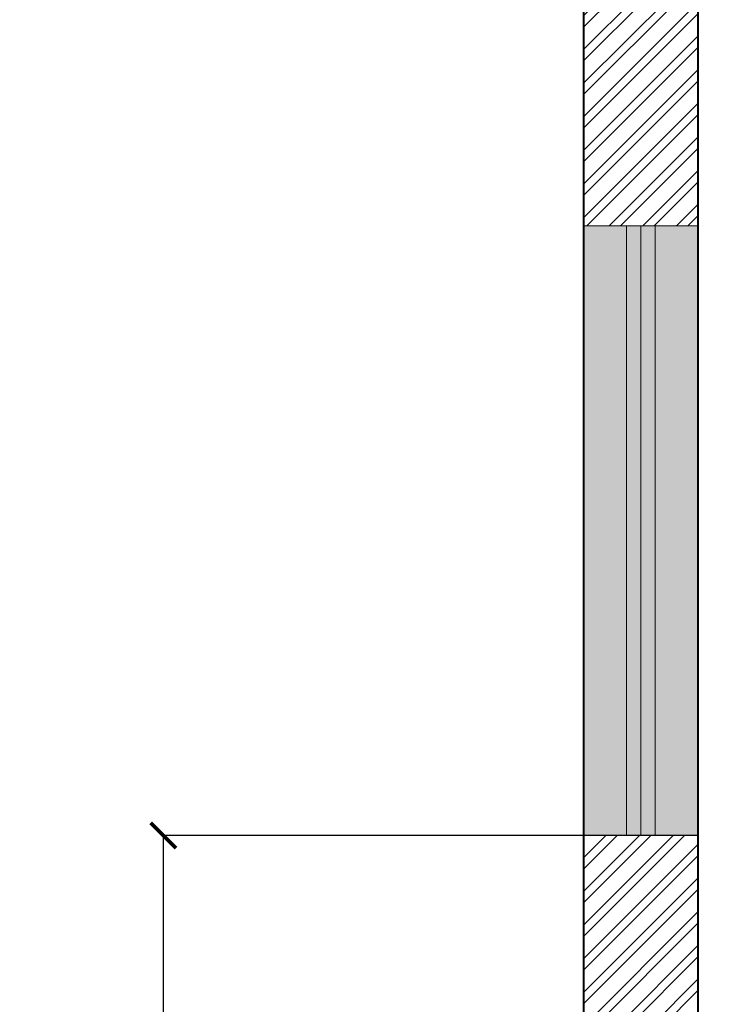
# Model space of a CAD drawing. Units: inches. Extents: x 528 to 2520, y -151 to 1354.
# Tile 17 of 41: x 1079 to 1136, y 1151 to 1228. Entities that reach past the tile are written whole.
import ezdxf

# ---------------------------------------------------------------- set-up
doc = ezdxf.new("R2010")
doc.units = ezdxf.units.IN
doc.header["$MEASUREMENT"] = 0
for name, color, linetype, lineweight in [('A-ANNO-DIMS', 2, 'Continuous', 18), ('A-WALL-PATT', 6, 'Continuous', 13), ('walls', 7, 'Continuous', 40), ('WINDOWS', 2, 'Continuous', 20)]:
    doc.layers.add(name, color=color, linetype=linetype, lineweight=lineweight)
doc.layers.add('A-GLAZ-PATT', color=152, linetype='Continuous', lineweight=13, true_color=0x2776bb)
doc.styles.get("Standard").update_dxf_attribs({"font": 'arial.ttf'})
doc.dimstyles.get("Standard").update_dxf_attribs({"dimtxt": 6, "dimasz": 2, "dimexe": 0.18, "dimexo": 0.0625, "dimgap": 0.09, "dimtad": 0, "dimtih": 1, "dimtoh": 1, "dimdec": 1, "dimzin": 0, "dimdsep": 46, "dimlunit": 3, "dimtxsty": 'Standard', "dimblk": 'ARCHTICK', "dimcen": 0.09, "dimadec": 0, "dimazin": 0, "dimtfac": 1, "dimtdec": 1, "dimtofl": 0, "dimtmove": 0, "dimatfit": 3, "dimfxl": 1, "dimtolj": 1, "dimtzin": 0, "dimarcsym": 0})

# ---------------------------------------------------------------- blocks, each defined once
blk = doc.blocks.new('WINDOW-48x9-PLAN')
for p, q in [((0, 5.632), (48, 5.632)), ((0, 4.5), (48, 4.5)), ((0, 3.368), (48, 3.368))]:
    blk.add_line(p, q)
blk.add_lwpolyline([(0, 9), (48, 9), (48, 0), (0, 0)], close=True)
blk = doc.blocks.new('_ArchTick')
at = {"color": 0, "linetype": 'ByBlock', "const_width": 0.15}
blk.add_lwpolyline([(-0.5, -0.5), (0.5, 0.5)], dxfattribs=at)
blk = doc.blocks.new('*D99')
at = {"layer": 'A-ANNO-DIMS', "color": 0, "lineweight": -2, "transparency": 16777216}
for p, q in [((1132.821, 1163.855), (1090.603, 1163.855)), ((1090.783, 1163.855), (1090.783, 1126.132)), ((1090.783, 1082.103), (1090.783, 1119.826)), ((1132.821, 1082.103), (1090.603, 1082.103))]:
    blk.add_line(p, q, dxfattribs=at)
at = {"layer": 'Defpoints', "color": 0, "transparency": 16777216}
for p in [(1132.883, 1163.855), (1090.783, 1082.103), (1132.883, 1082.103)]:
    blk.add_point(p, dxfattribs=at)
at = {"layer": 'A-ANNO-DIMS', "color": 0, "lineweight": -2, "transparency": 16777216, "xscale": 2, "yscale": 2, "zscale": 2}
for p, rotation in [((1090.783, 1163.855), 90), ((1090.783, 1082.103), 270)]:
    blk.add_blockref('_ArchTick', p, dxfattribs=dict(at, rotation=rotation))
at = {"layer": 'A-ANNO-DIMS', "color": 0, "transparency": 16777216, "insert": (1090.783, 1122.979), "char_height": 6, "attachment_point": 5}
blk.add_mtext('\\A1;6\'-10"', dxfattribs=at)

msp = doc.modelspace()

# ---------------------------------------------------------------- hatches: boundary and pattern name
at = {"layer": 'A-GLAZ-PATT'}
h = msp.add_hatch(color=256, dxfattribs=at)
h.dxf.hatch_style = 1
h.paths.add_polyline_path([(1123.883, 1211.855), (1123.883, 1163.855), (1127.252, 1163.855), (1127.252, 1211.855)])
h.paths.add_polyline_path([(1127.252, 1211.855), (1127.252, 1163.855), (1128.383, 1163.855), (1128.383, 1211.855)])
h.paths.add_polyline_path([(1128.383, 1211.855), (1128.383, 1163.855), (1129.515, 1163.855), (1129.515, 1211.855)])
h.paths.add_polyline_path([(1129.515, 1211.855), (1129.515, 1163.855), (1132.883, 1163.855), (1132.883, 1211.855)])
at = {"layer": 'A-WALL-PATT'}
h = msp.add_hatch(dxfattribs=at)
h.set_pattern_fill('ANSI32', color=256, scale=5)
h.set_pattern_definition([(45, (537.1868, 0), (-1.3258252, 1.3258252), []), (45, (538.0707, 0), (-1.3258252, 1.3258252), [])])
h.paths.add_polyline_path([(1132.883, 1163.855), (1123.883, 1163.855), (1123.883, 969.103), (1135.43, 969.103), (1140.43, 969.103), (1140.43, 974.103), (1132.883, 974.103), (1132.883, 1082.103), (1228.883, 1082.103), (1228.883, 1087.103), (1228.883, 1106.103), (1234.883, 1106.103), (1234.883, 1111.103), (1223.883, 1111.103), (1223.883, 1087.103), (1132.883, 1087.103)])
h.paths.add_polyline_path([(1225.889, 974.103), (1188.43, 974.103), (1188.43, 969.103), (1225.889, 969.103)])
h.paths.add_polyline_path([(1422.883, 1171.369), (1413.883, 1171.369), (1413.883, 1111.103), (1323.883, 1111.103), (1323.883, 1106.103), (1413.883, 1106.103), (1413.883, 974.103), (1323.883, 974.103), (1323.883, 969.103), (1413.883, 969.103), (1413.883, 825.103), (1371.883, 825.103), (1371.883, 816.103), (1422.883, 816.103)])
h.paths.add_polyline_path([(1422.883, 1317.103), (1413.839, 1317.103), (1413.839, 1308.103), (1413.883, 1308.103), (1413.883, 1248.103), (1359.883, 1248.103), (1359.883, 1243.103), (1413.883, 1243.103), (1413.883, 1219.369), (1422.883, 1219.369)])
h.paths.add_polyline_path([(1389.839, 1317.103), (1324.883, 1317.103), (1324.883, 1248.103), (1321.45, 1248.103), (1321.45, 1243.103), (1329.883, 1243.103), (1329.883, 1249.103), (1329.883, 1308.103), (1389.839, 1308.103)])
h.paths.add_polyline_path([(1221.883, 1317.103), (1156.883, 1317.103), (1156.883, 1308.103), (1216.883, 1308.103), (1216.883, 1248.103), (1216.883, 1243.103), (1221.883, 1243.103), (1221.883, 1248.248)])
h.paths.add_polyline_path([(1132.883, 1308.103), (1132.883, 1317.103), (1123.883, 1317.103), (1123.883, 1211.855), (1132.883, 1211.855), (1132.883, 1243.103), (1186.883, 1243.103), (1186.883, 1248.103), (1132.883, 1248.103)])
h.paths.add_polyline_path([(1281.883, 969.103), (1281.883, 974.103), (1261.889, 974.103), (1261.889, 969.103), (1276.883, 969.103), (1276.883, 874.287), (1281.883, 874.287)])
h.paths.add_polyline_path([(1276.883, 969.103), (1264.883, 969.103), (1264.883, 965.117), (1267.922, 965.117), (1267.922, 961.676), (1271.621, 961.676), (1271.621, 957.24), (1276.883, 957.24)], flags=17)
h.paths.add_polyline_path([(1323.883, 825.103), (1281.883, 825.103), (1281.883, 832.287), (1276.883, 832.287), (1276.883, 816.103), (1323.883, 816.103)])

# ---------------------------------------------------------------- linework, layer by layer
at = {"layer": 'walls'}
for p, q in [((1123.883, 1317.103), (1123.883, 969.103)), ((1132.883, 1243.103), (1132.883, 1087.103))]:
    msp.add_line(p, q, dxfattribs=at)

# ---------------------------------------------------------------- block references
at = {"layer": 'WINDOWS', "rotation": 90.00000000000006}
msp.add_blockref('WINDOW-48x9-PLAN', (1132.883, 1163.856), dxfattribs=at)

# ---------------------------------------------------------------- dimensions: what is measured, and where the dimension line sits
at = {"layer": 'A-ANNO-DIMS'}
dim = msp.add_linear_dim(base=(1090.783, 1082.103), p1=(1132.883, 1163.855), p2=(1132.883, 1082.103), angle=90, dimstyle='Standard', override={"dimdec": 1, "dimlfac": 1, "dimrnd": 0, "dimzin": 1, "dimdsep": 46, "dimlunit": 4, "dimfrac": 2}, dxfattribs=at)
dim.commit()
dim.dimension.update_dxf_attribs({"geometry": '*D99', "text_midpoint": (1090.783, 1122.979)})

doc.saveas('drawing.dxf')
